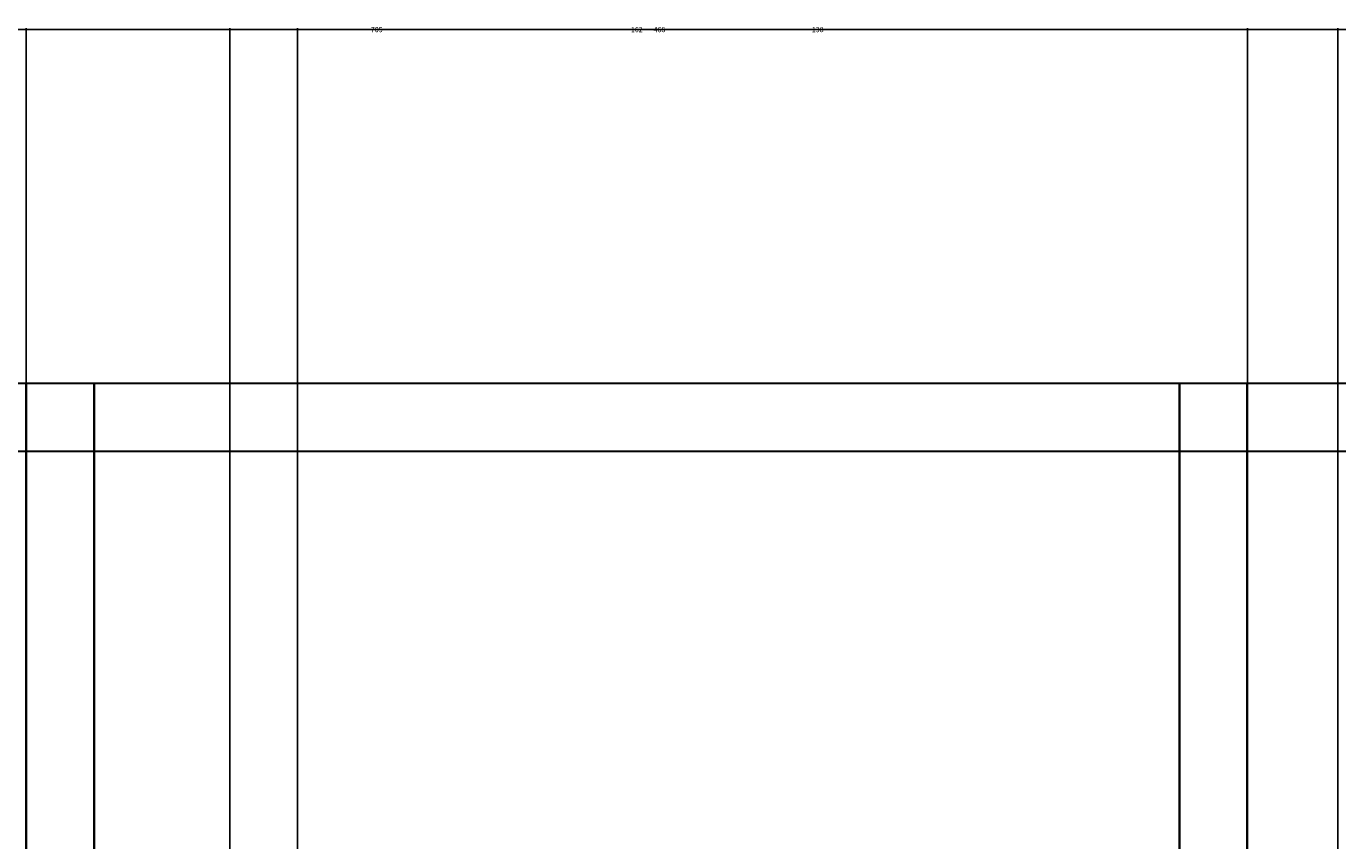
# Model space of a CAD drawing. Units: inches. Extents: x 867 to 1667, y -234 to 788.
# Tile 35 of 42: x 1221 to 1395, y 680 to 788. Entities that reach past the tile are written whole.
import ezdxf

# ---------------------------------------------------------------- set-up
doc = ezdxf.new("R2010")
doc.units = ezdxf.units.IN
doc.header["$MEASUREMENT"] = 0
for name, color, linetype, lineweight in [('A-ANNO-DIMS', 2, 'Continuous', 18), ('A-Wall', 7, 'Continuous', 35), ('A-WALL-SITE', 8, 'Continuous', 30)]:
    doc.layers.add(name, color=color, linetype=linetype, lineweight=lineweight)
doc.styles.get("Standard").update_dxf_attribs({"font": 'arial.ttf'})
doc.dimstyles.get("Standard").update_dxf_attribs({"dimtxt": 0.6875, "dimasz": 0.18, "dimexe": 0.18, "dimexo": 0.0625, "dimgap": 0.09, "dimtad": 0, "dimdec": 4, "dimzin": 0, "dimdsep": 46, "dimlunit": 4, "dimtxsty": 'Standard', "dimcen": 0.09, "dimadec": 0, "dimazin": 0, "dimtfac": 1, "dimtdec": 4, "dimtofl": 0, "dimtmove": 0, "dimatfit": 3, "dimfxl": 1, "dimtolj": 1, "dimtzin": 0, "dimarcsym": 0})

# ---------------------------------------------------------------- blocks, each defined once
blk = doc.blocks.new('*D17')
at = {"layer": 'A-ANNO-DIMS', "color": 0, "lineweight": -2, "transparency": 16777216}
for p, q in [((914.89, 740.68), (914.89, 787.75)), ((915.07, 787.57), (1266.54, 787.57)), ((1619.71, 787.57), (1268.24, 787.57)), ((1619.89, 740.68), (1619.89, 787.75))]:
    blk.add_line(p, q, dxfattribs=at)
at = {"layer": 'A-ANNO-DIMS', "color": 0, "transparency": 16777216}
for points in [[(915.07, 787.6), (915.07, 787.54), (914.89, 787.57)], [(1619.71, 787.6), (1619.71, 787.54), (1619.89, 787.57)]]:
    blk.add_solid(points, dxfattribs=at)
at = {"layer": 'Defpoints', "color": 0, "transparency": 16777216}
for p in [(1619.89, 787.57), (914.89, 740.62), (1619.89, 740.62)]:
    blk.add_point(p, dxfattribs=at)
at = {"layer": 'A-ANNO-DIMS', "color": 0, "transparency": 16777216, "insert": (1267.39, 787.57), "char_height": 0.688, "attachment_point": 5}
blk.add_mtext('\\A1;705', dxfattribs=at)
blk = doc.blocks.new('*D22')
at = {"layer": 'A-ANNO-DIMS', "color": 0, "lineweight": -2, "transparency": 16777216}
for p, q in [((1220.89, 740.68), (1220.89, 787.75)), ((1221.07, 787.57), (1301.07, 787.57)), ((1382.71, 787.57), (1302.7, 787.57)), ((1382.89, 740.68), (1382.89, 787.75))]:
    blk.add_line(p, q, dxfattribs=at)
at = {"layer": 'A-ANNO-DIMS', "color": 0, "transparency": 16777216}
for points in [[(1221.07, 787.6), (1221.07, 787.54), (1220.89, 787.57)], [(1382.71, 787.6), (1382.71, 787.54), (1382.89, 787.57)]]:
    blk.add_solid(points, dxfattribs=at)
at = {"layer": 'Defpoints', "color": 0, "transparency": 16777216}
for p in [(1382.89, 787.57), (1220.89, 740.62), (1382.89, 740.62)]:
    blk.add_point(p, dxfattribs=at)
at = {"layer": 'A-ANNO-DIMS', "color": 0, "transparency": 16777216, "insert": (1301.89, 787.57), "char_height": 0.688, "attachment_point": 5}
blk.add_mtext('\\A1;162', dxfattribs=at)
blk = doc.blocks.new('*D31')
at = {"layer": 'A-ANNO-DIMS', "color": 0, "lineweight": -2, "transparency": 16777216}
for p, q in [((1070.89, 566.68), (1070.89, 787.75)), ((1071.07, 787.57), (1304.02, 787.57)), ((1538.71, 787.57), (1305.75, 787.57)), ((1538.89, 566.68), (1538.89, 787.75))]:
    blk.add_line(p, q, dxfattribs=at)
at = {"layer": 'A-ANNO-DIMS', "color": 0, "transparency": 16777216}
for points in [[(1071.07, 787.6), (1071.07, 787.54), (1070.89, 787.57)], [(1538.71, 787.6), (1538.71, 787.54), (1538.89, 787.57)]]:
    blk.add_solid(points, dxfattribs=at)
at = {"layer": 'Defpoints', "color": 0, "transparency": 16777216}
for p in [(1538.89, 787.57), (1070.89, 566.62), (1538.89, 566.62)]:
    blk.add_point(p, dxfattribs=at)
at = {"layer": 'A-ANNO-DIMS', "color": 0, "transparency": 16777216, "insert": (1304.89, 787.57), "char_height": 0.688, "attachment_point": 5}
blk.add_mtext('\\A1;468', dxfattribs=at)
blk = doc.blocks.new('*D32')
at = {"layer": 'A-ANNO-DIMS', "color": 0, "lineweight": -2, "transparency": 16777216}
for p, q in [((1079.89, 404.68), (1079.89, 787.75)), ((1080.07, 787.57), (1163.07, 787.57)), ((1247.71, 787.57), (1164.7, 787.57)), ((1247.89, 413.68), (1247.89, 787.75))]:
    blk.add_line(p, q, dxfattribs=at)
at = {"layer": 'A-ANNO-DIMS', "color": 0, "transparency": 16777216}
for points in [[(1080.07, 787.6), (1080.07, 787.54), (1079.89, 787.57)], [(1247.71, 787.6), (1247.71, 787.54), (1247.89, 787.57)]]:
    blk.add_solid(points, dxfattribs=at)
at = {"layer": 'Defpoints', "color": 0, "transparency": 16777216}
for p in [(1247.89, 787.57), (1247.89, 413.62), (1079.89, 404.62)]:
    blk.add_point(p, dxfattribs=at)
at = {"layer": 'A-ANNO-DIMS', "color": 0, "transparency": 16777216, "insert": (1163.89, 787.57), "char_height": 0.688, "attachment_point": 5}
blk.add_mtext('\\A1;168', dxfattribs=at)
blk = doc.blocks.new('*D33')
at = {"layer": 'A-ANNO-DIMS', "color": 0, "lineweight": -2, "transparency": 16777216}
for p, q in [((1256.89, 413.68), (1256.89, 787.75)), ((1257.07, 787.57), (1325.07, 787.57)), ((1394.71, 787.57), (1326.7, 787.57)), ((1394.89, 413.68), (1394.89, 787.75))]:
    blk.add_line(p, q, dxfattribs=at)
at = {"layer": 'A-ANNO-DIMS', "color": 0, "transparency": 16777216}
for points in [[(1257.07, 787.6), (1257.07, 787.54), (1256.89, 787.57)], [(1394.71, 787.6), (1394.71, 787.54), (1394.89, 787.57)]]:
    blk.add_solid(points, dxfattribs=at)
at = {"layer": 'Defpoints', "color": 0, "transparency": 16777216}
for p in [(1394.89, 787.57), (1256.89, 413.62), (1394.89, 413.62)]:
    blk.add_point(p, dxfattribs=at)
at = {"layer": 'A-ANNO-DIMS', "color": 0, "transparency": 16777216, "insert": (1325.89, 787.57), "char_height": 0.688, "attachment_point": 5}
blk.add_mtext('\\A1;138', dxfattribs=at)

msp = doc.modelspace()

# ---------------------------------------------------------------- linework, layer by layer
at = {"layer": 'A-Wall'}
for p, q in [((1220.8866, 740.617), (1220.8866, 623.617)), ((1229.8866, 740.617), (1229.8866, 623.617)), ((1373.8866, 740.617), (1373.8866, 623.617)), ((1382.8866, 740.617), (1382.8866, 623.617))]:
    msp.add_line(p, q, dxfattribs=at)
at = {"layer": 'A-WALL-SITE'}
for p, q in [((1619.8866, 740.617), (914.8866, 740.617)), ((1619.8866, 731.617), (914.8866, 731.617))]:
    msp.add_line(p, q, dxfattribs=at)

# ---------------------------------------------------------------- dimensions: what is measured, and where the dimension line sits
at = {"layer": 'A-ANNO-DIMS'}
for base, p1, p2, picture, middle in [((1619.8866, 787.567), (914.8866, 740.617), (1619.8866, 740.617), '*D17', (1267.3866, 787.567)), ((1538.8866, 787.567), (1070.8866, 566.617), (1538.8866, 566.617), '*D31', (1304.8866, 787.567)), ((1247.8866, 787.567), (1079.8866, 404.617), (1247.8866, 413.617), '*D32', (1163.8866, 787.567)), ((1382.8866, 787.567), (1220.8866, 740.617), (1382.8866, 740.617), '*D22', (1301.8866, 787.567)), ((1394.8866, 787.567), (1256.8866, 413.617), (1394.8866, 413.617), '*D33', (1325.8866, 787.567))]:
    dim = msp.add_linear_dim(base=base, p1=p1, p2=p2, dimstyle='Standard', override={"dimdec": 0, "dimlfac": 1, "dimrnd": 0, "dimzin": 0, "dimdsep": 46, "dimlunit": 2}, dxfattribs=at)
    dim.commit()
    dim.dimension.update_dxf_attribs({"geometry": picture, "text_midpoint": middle})

doc.saveas('drawing.dxf')
